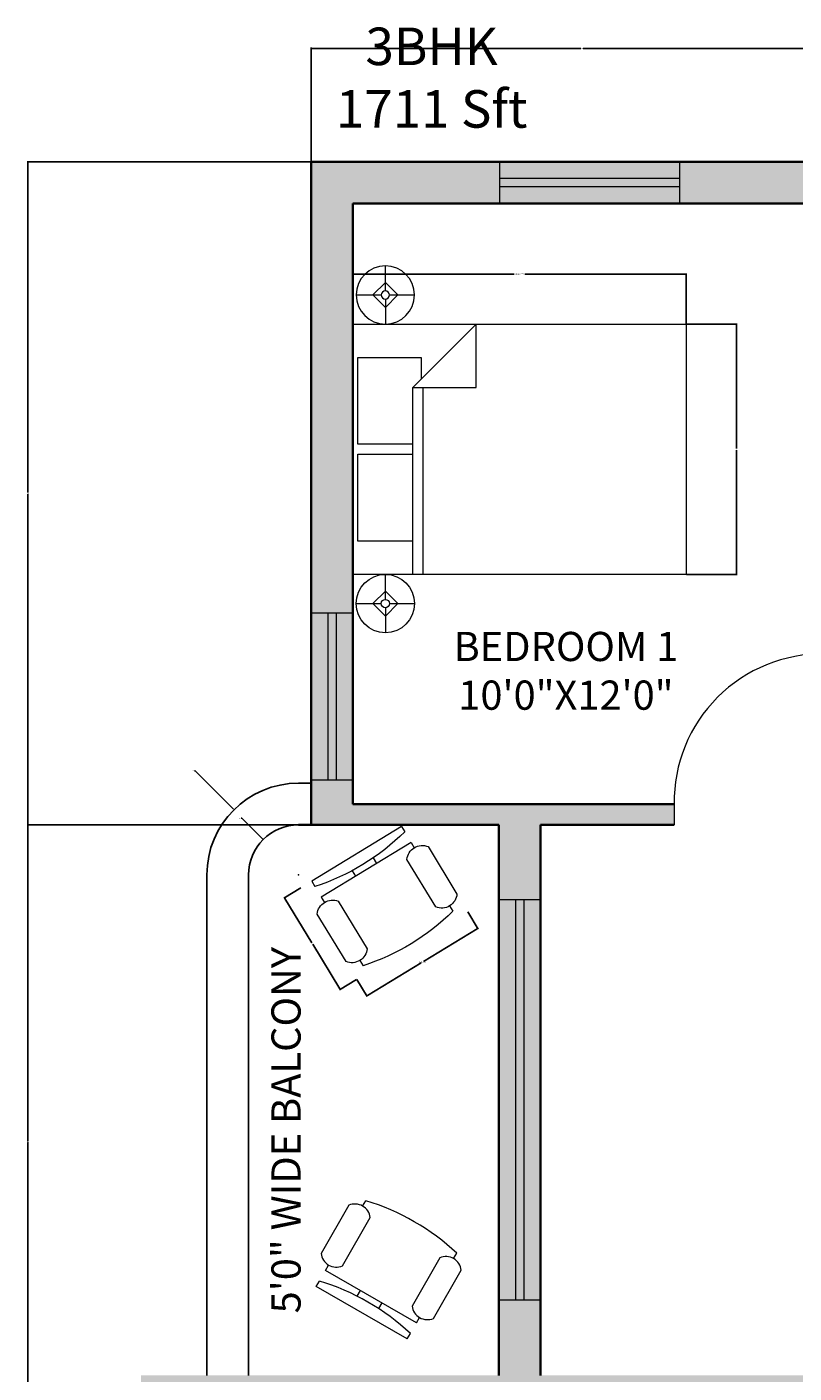
# Model space of a CAD drawing. Units: inches. Extents: x -382 to 250, y 518 to 1732.
# Tile 6 of 8: x -270 to -86, y 1373 to 1695. Entities that reach past the tile are written whole.
import ezdxf

# ---------------------------------------------------------------- set-up
doc = ezdxf.new("R2010")
doc.units = ezdxf.units.IN
doc.header["$MEASUREMENT"] = 0
for name, color, linetype, lineweight in [('A-ANNO-DIMS', 2, 'Continuous', 18), ('A-ANNO-TEXT', 7, 'Continuous', 25), ('A-AREA-IDEN', 7, 'Continuous', 18), ('A-DOOR', 3, 'Continuous', 18), ('A-FLOR-EDGE', 7, 'Continuous', 25), ('A-FURN', 8, 'Continuous', 18), ('A-GLAZ', 4, 'Continuous', 18), ('A-WALL', 7, 'Continuous', 35)]:
    doc.layers.add(name, color=color, linetype=linetype, lineweight=lineweight)
doc.layers.add('A-GLAZ-PATT', color=143, linetype='Continuous', lineweight=13, true_color=0x7aafdf)
doc.layers.add('A-WALL-PATT', color=251, linetype='Continuous', lineweight=13, true_color=0x636466)
doc.styles.get("Standard").update_dxf_attribs({"font": 'arial.ttf'})
doc.dimstyles.get("Standard").update_dxf_attribs({"dimtxt": 0.18, "dimasz": 0.18, "dimexe": 0.18, "dimexo": 0.0625, "dimgap": 0.09, "dimtad": 0, "dimtih": 1, "dimtoh": 1, "dimdec": 4, "dimzin": 0, "dimdsep": 46, "dimtxsty": 'Standard', "dimcen": 0.09, "dimadec": 0, "dimazin": 0, "dimtfac": 1, "dimtdec": 4, "dimtofl": 0, "dimtmove": 0, "dimatfit": 3, "dimfxl": 1, "dimtolj": 1, "dimtzin": 0, "dimarcsym": 0})

# ---------------------------------------------------------------- blocks, each defined once
blk = doc.blocks.new('Bed - Queen')
for p, q in [((0, -80.00003), (0, 0)), ((0, 0), (59.99999, 0)), ((59.99999, 0), (59.99999, -80.00003)), ((7.99999, -1.2), (28.79998, -1.2)), ((7.99999, -14.4), (7.99999, -1.2)), ((28.79998, -1.2), (28.79998, -14.4)), ((31.19999, -1.2), (51.99999, -1.2)), ((31.19999, -14.4), (31.19999, -1.2)), ((51.99999, -1.2), (51.99999, -16.4)), ((0, -14.4), (44.8, -14.4)), ((59.99999, -29.6), (44.8, -14.4)), ((44.8, -14.4), (44.8, -29.6)), ((44.8, -16.8), (0, -16.8)), ((51.99999, -16.4), (46.79936, -16.4)), ((44.8, -29.6), (59.99999, -29.6)), ((59.99999, -80.00003), (0, -80.00003))]:
    blk.add_line(p, q)
blk = doc.blocks.new('Lamp - Table')
for p, q in [((0, 7), (0, 1)), ((-1, 0), (-7, 0)), ((0, 3), (-3, 0)), ((-3, 0), (0, -3)), ((3, 0), (0, 3)), ((0, -3), (3, 0)), ((1, 0), (7, 0)), ((0, -1), (0, -7))]:
    blk.add_line(p, q)
for radius in [7, 1]:
    blk.add_circle((0, 0), radius)
blk = doc.blocks.new('Chair - Desk')
for p, q in [((-8.5, 0), (-8.5, -1)), ((-8.5, 0), (8.5, 0)), ((8.5, 0), (8.5, -1)), ((-2, -3), (-2, -1.9355)), ((2, -1.9576), (2, -3)), ((-8.5, -3), (-8.5, -4)), ((-8.5, -3), (8.5, -3)), ((8.5, -3), (8.5, -4)), ((-10.5, -5), (-10.5, -14)), ((-6.5, -14), (-6.5, -5)), ((6.5, -5), (6.5, -14)), ((10.5, -14), (10.5, -5)), ((-8.5, -15), (-8.5, -16)), ((8.5, -15), (8.5, -16))]:
    blk.add_line(p, q)
for centre, radius, start, end in [((0, 34.625), 36.625, 256.5803, 283.4197), ((-8.5, -6.5), 2.5, 36.8699, 143.1301), ((8.5, -6.5), 2.5, 36.8699, 143.1301), ((-8.5, -12.5), 2.5, 216.8699, 323.1301), ((8.5, -12.5), 2.5, 216.8699, 323.1301), ((0, 19.625), 36.625, 256.5803, 283.4197)]:
    blk.add_arc(centre, radius, start, end)
blk = doc.blocks.new('WIN-43_2IN')
for p, q in [((0, 10), (0, 0)), ((43.2, 10), (43.2, 0)), ((0, 6), (43.2, 6)), ((0, 4), (43.2, 4))]:
    blk.add_line(p, q)
blk = doc.blocks.new('WIN-40IN')
for p, q in [((10, 40), (0, 40)), ((4, 40), (4, 0)), ((6, 40), (6, 0)), ((10, 0), (0, 0))]:
    blk.add_line(p, q)
blk = doc.blocks.new('DOOR-SWING-36IN')
for p, q in [((-1, 0), (-1, 36)), ((0, 0), (0, 36))]:
    blk.add_line(p, q)
blk.add_arc((-0.5, 0.5), 35.5, 89.1931, 180.8069)
blk = doc.blocks.new('GLAZ-BALCONY-96IN')
for p, q in [((0, 10), (0, 0)), ((96, 10), (96, 0)), ((0, 6), (96, 6)), ((0, 4), (96, 4))]:
    blk.add_line(p, q)
blk = doc.blocks.new('*D28')
at = {"layer": 'A-ANNO-DIMS', "color": 0, "lineweight": -2, "transparency": 16777216}
for p, q in [((-192.22, 1624.2), (-192.22, 1636.31)), ((-192.04, 1636.13), (-153.52, 1636.13)), ((-112.39, 1636.13), (-150.91, 1636.13)), ((-112.21, 1624.2), (-112.21, 1636.31))]:
    blk.add_line(p, q, dxfattribs=at)
at = {"layer": 'A-ANNO-DIMS', "color": 0, "transparency": 16777216}
for points in [[(-192.04, 1636.16), (-192.04, 1636.1), (-192.22, 1636.13)], [(-112.39, 1636.16), (-112.39, 1636.1), (-112.21, 1636.13)]]:
    blk.add_solid(points, dxfattribs=at)
at = {"layer": 'Defpoints', "color": 0, "transparency": 16777216}
for p in [(-192.22, 1636.13), (-192.22, 1624.13), (-112.21, 1624.13)]:
    blk.add_point(p, dxfattribs=at)
at = {"layer": 'A-ANNO-DIMS', "color": 0, "transparency": 16777216, "insert": (-152.22, 1636.13), "char_height": 0.18, "attachment_point": 5}
blk.add_mtext('\\A1;QUEEN BED 80 TYP.', dxfattribs=at)
blk = doc.blocks.new('*D29')
at = {"layer": 'A-ANNO-DIMS', "color": 0, "lineweight": -2, "transparency": 16777216}
for p, q in [((-112.15, 1624.13), (-100.03, 1624.13)), ((-100.21, 1623.95), (-100.21, 1594.32)), ((-100.21, 1564.31), (-100.21, 1593.95)), ((-112.15, 1564.13), (-100.03, 1564.13))]:
    blk.add_line(p, q, dxfattribs=at)
at = {"layer": 'A-ANNO-DIMS', "color": 0, "transparency": 16777216}
for points in [[(-100.24, 1623.95), (-100.18, 1623.95), (-100.21, 1624.13)], [(-100.24, 1564.31), (-100.18, 1564.31), (-100.21, 1564.13)]]:
    blk.add_solid(points, dxfattribs=at)
at = {"layer": 'Defpoints', "color": 0, "transparency": 16777216}
for p in [(-112.21, 1624.13), (-100.21, 1624.13), (-112.21, 1564.13)]:
    blk.add_point(p, dxfattribs=at)
at = {"layer": 'A-ANNO-DIMS', "color": 0, "transparency": 16777216, "insert": (-100.21, 1594.13), "char_height": 0.18, "attachment_point": 5}
blk.add_mtext('\\A1;60 TYP.', dxfattribs=at)
blk = doc.blocks.new('*D38')
at = {"layer": 'A-ANNO-DIMS', "color": 0, "lineweight": -2, "transparency": 16777216}
for p, q in [((-164.62, 1483.19), (-162.13, 1479.09)), ((-162.38, 1479.15), (-175.23, 1471.34)), ((-188.68, 1463.16), (-175.83, 1470.98)), ((-191.22, 1467.01), (-188.74, 1462.92))]:
    blk.add_line(p, q, dxfattribs=at)
at = {"layer": 'A-ANNO-DIMS', "color": 0, "transparency": 16777216}
for points in [[(-162.4, 1479.18), (-162.36, 1479.13), (-162.23, 1479.25)], [(-188.69, 1463.19), (-188.66, 1463.14), (-188.83, 1463.07)]]:
    blk.add_solid(points, dxfattribs=at)
at = {"layer": 'Defpoints', "color": 0, "transparency": 16777216}
for p in [(-164.65, 1483.24), (-191.26, 1467.06), (-188.83, 1463.07)]:
    blk.add_point(p, dxfattribs=at)
at = {"layer": 'A-ANNO-DIMS', "color": 0, "transparency": 16777216, "insert": (-175.53, 1471.16), "char_height": 0.18, "attachment_point": 5}
blk.add_mtext('\\A1;CHAIR 31 TYP.', dxfattribs=at)
blk = doc.blocks.new('*D39')
at = {"layer": 'A-ANNO-DIMS', "color": 0, "lineweight": -2, "transparency": 16777216}
for p, q in [((-204.66, 1488.99), (-208.75, 1486.5)), ((-208.51, 1486.44), (-202.03, 1475.8)), ((-195.34, 1464.79), (-201.81, 1475.43)), ((-191.31, 1467.03), (-195.4, 1464.54))]:
    blk.add_line(p, q, dxfattribs=at)
at = {"layer": 'A-ANNO-DIMS', "color": 0, "transparency": 16777216}
for points in [[(-208.48, 1486.46), (-208.53, 1486.42), (-208.6, 1486.59)], [(-195.32, 1464.8), (-195.37, 1464.77), (-195.25, 1464.63)]]:
    blk.add_solid(points, dxfattribs=at)
at = {"layer": 'Defpoints', "color": 0, "transparency": 16777216}
for p in [(-204.61, 1489.02), (-208.6, 1486.59), (-191.26, 1467.06)]:
    blk.add_point(p, dxfattribs=at)
at = {"layer": 'A-ANNO-DIMS', "color": 0, "transparency": 16777216, "insert": (-201.92, 1475.61), "char_height": 0.18, "attachment_point": 5}
blk.add_mtext('\\A1;26 TYP.', dxfattribs=at)
blk = doc.blocks.new('*D88')
at = {"layer": 'A-ANNO-DIMS', "color": 0, "lineweight": -2, "transparency": 16777216}
for p, q in [((-202.22, 1663.13), (-202.22, 1690.45)), ((-202.04, 1690.27), (-137.5, 1690.27)), ((-72.4, 1690.27), (-136.93, 1690.27)), ((-72.22, 1663.13), (-72.22, 1690.45))]:
    blk.add_line(p, q, dxfattribs=at)
at = {"layer": 'A-ANNO-DIMS', "color": 0, "transparency": 16777216}
for points in [[(-202.04, 1690.3), (-202.04, 1690.24), (-202.22, 1690.27)], [(-72.4, 1690.3), (-72.4, 1690.24), (-72.22, 1690.27)]]:
    blk.add_solid(points, dxfattribs=at)
at = {"layer": 'Defpoints', "color": 0, "transparency": 16777216}
for p in [(-72.22, 1690.27), (-202.22, 1663.07), (-72.22, 1663.07)]:
    blk.add_point(p, dxfattribs=at)
at = {"layer": 'A-ANNO-DIMS', "color": 0, "transparency": 16777216, "insert": (-137.22, 1690.27), "char_height": 0.18, "attachment_point": 5}
blk.add_mtext('\\A1;130', dxfattribs=at)
blk = doc.blocks.new('*D92')
at = {"layer": 'A-ANNO-DIMS', "color": 0, "lineweight": -2, "transparency": 16777216}
for p, q in [((-202.28, 1504.07), (-270.36, 1504.07)), ((-270.18, 1503.89), (-270.18, 1428.25)), ((-270.18, 1352.25), (-270.18, 1427.89)), ((-243.04, 1352.07), (-270.36, 1352.07))]:
    blk.add_line(p, q, dxfattribs=at)
at = {"layer": 'A-ANNO-DIMS', "color": 0, "transparency": 16777216}
for points in [[(-270.21, 1503.89), (-270.15, 1503.89), (-270.18, 1504.07)], [(-270.21, 1352.25), (-270.15, 1352.25), (-270.18, 1352.07)]]:
    blk.add_solid(points, dxfattribs=at)
at = {"layer": 'Defpoints', "color": 0, "transparency": 16777216}
for p in [(-270.18, 1504.07), (-202.22, 1504.07), (-242.98, 1352.07)]:
    blk.add_point(p, dxfattribs=at)
at = {"layer": 'A-ANNO-DIMS', "color": 0, "transparency": 16777216, "insert": (-270.18, 1428.07), "char_height": 0.18, "attachment_point": 5}
blk.add_mtext('\\A1;152', dxfattribs=at)
blk = doc.blocks.new('*D93')
at = {"layer": 'A-ANNO-DIMS', "color": 0, "lineweight": -2, "transparency": 16777216}
for p, q in [((-202.28, 1663.07), (-270.36, 1663.07)), ((-270.18, 1662.89), (-270.18, 1583.75)), ((-270.18, 1504.25), (-270.18, 1583.39)), ((-202.28, 1504.07), (-270.36, 1504.07))]:
    blk.add_line(p, q, dxfattribs=at)
at = {"layer": 'A-ANNO-DIMS', "color": 0, "transparency": 16777216}
for points in [[(-270.21, 1662.89), (-270.15, 1662.89), (-270.18, 1663.07)], [(-270.21, 1504.25), (-270.15, 1504.25), (-270.18, 1504.07)]]:
    blk.add_solid(points, dxfattribs=at)
at = {"layer": 'Defpoints', "color": 0, "transparency": 16777216}
for p in [(-270.18, 1663.07), (-202.22, 1663.07), (-202.22, 1504.07)]:
    blk.add_point(p, dxfattribs=at)
at = {"layer": 'A-ANNO-DIMS', "color": 0, "transparency": 16777216, "insert": (-270.18, 1583.57), "char_height": 0.18, "attachment_point": 5}
blk.add_mtext('\\A1;159', dxfattribs=at)
blk = doc.blocks.new('*D98')
at = {"layer": 'A-ANNO-DIMS', "color": 0, "lineweight": -2, "transparency": 16777216}
for p, q in [((-230.17, 1517.07), (-229.99, 1517.07)), ((-229.99, 1517.07), (-220.83, 1507.82)), ((-205.31, 1492.07), (-205.13, 1492.07)), ((-205.22, 1491.98), (-205.22, 1492.16))]:
    blk.add_line(p, q, dxfattribs=at)
at = {"layer": 'A-ANNO-DIMS', "color": 0, "transparency": 16777216}
blk.add_solid([(-220.8, 1507.85), (-220.85, 1507.8), (-220.7, 1507.7)], dxfattribs=at)
at = {"layer": 'Defpoints', "color": 0, "transparency": 16777216}
for p in [(-220.7, 1507.7), (-205.22, 1492.07)]:
    blk.add_point(p, dxfattribs=at)
at = {"layer": 'A-ANNO-DIMS', "color": 0, "transparency": 16777216, "insert": (-230.47, 1517.07), "char_height": 0.18, "attachment_point": 5}
blk.add_mtext('\\A1;R22', dxfattribs=at)
blk = doc.blocks.new('*D99')
at = {"layer": 'A-ANNO-DIMS', "color": 0, "lineweight": -2, "transparency": 16777216}
for p, q in [((-218.97, 1505.65), (-218.79, 1505.65)), ((-218.79, 1505.65), (-213.83, 1500.68)), ((-205.31, 1492.07), (-205.13, 1492.07)), ((-205.22, 1491.98), (-205.22, 1492.16))]:
    blk.add_line(p, q, dxfattribs=at)
at = {"layer": 'A-ANNO-DIMS', "color": 0, "transparency": 16777216}
blk.add_solid([(-213.81, 1500.7), (-213.85, 1500.66), (-213.7, 1500.55)], dxfattribs=at)
at = {"layer": 'Defpoints', "color": 0, "transparency": 16777216}
for p in [(-213.7, 1500.55), (-205.22, 1492.07)]:
    blk.add_point(p, dxfattribs=at)
at = {"layer": 'A-ANNO-DIMS', "color": 0, "transparency": 16777216, "insert": (-219.28, 1505.65), "char_height": 0.18, "attachment_point": 5}
blk.add_mtext('\\A1;R12', dxfattribs=at)

msp = doc.modelspace()

# ---------------------------------------------------------------- hatches: boundary and pattern name
at = {"layer": 'A-GLAZ-PATT'}
h = msp.add_hatch(color=256, dxfattribs=at)
h.dxf.hatch_style = 1
h.paths.add_polyline_path([(-113.7732, 1663.0687), (-156.9732, 1663.0687), (-156.9732, 1659.0687), (-113.7732, 1659.0687)])
h = msp.add_hatch(color=256, dxfattribs=at)
h.dxf.hatch_style = 1
h.paths.add_polyline_path([(-113.7732, 1659.0687), (-156.9732, 1659.0687), (-156.9732, 1657.0687), (-113.7732, 1657.0687)])
h = msp.add_hatch(color=256, dxfattribs=at)
h.dxf.hatch_style = 1
h.paths.add_polyline_path([(-113.7732, 1657.0687), (-156.9732, 1657.0687), (-156.9732, 1653.0687), (-113.7732, 1653.0687)])
h = msp.add_hatch(color=256, dxfattribs=at)
h.dxf.hatch_style = 1
h.paths.add_polyline_path([(-198.215, 1554.8323), (-202.215, 1554.8323), (-202.215, 1514.8323), (-198.215, 1514.8323)])
h = msp.add_hatch(color=256, dxfattribs=at)
h.dxf.hatch_style = 1
h.paths.add_polyline_path([(-196.215, 1554.8323), (-198.215, 1554.8323), (-198.215, 1514.8323), (-196.215, 1514.8323)])
h = msp.add_hatch(color=256, dxfattribs=at)
h.dxf.hatch_style = 1
h.paths.add_polyline_path([(-192.215, 1554.8323), (-196.215, 1554.8323), (-196.215, 1514.8323), (-192.215, 1514.8323)])
h = msp.add_hatch(color=256, dxfattribs=at)
h.dxf.hatch_style = 1
h.paths.add_polyline_path([(-153.215, 1486.0687), (-157.215, 1486.0687), (-157.215, 1390.0687), (-153.215, 1390.0687)])
h = msp.add_hatch(color=256, dxfattribs=at)
h.dxf.hatch_style = 1
h.paths.add_polyline_path([(-151.215, 1486.0687), (-153.215, 1486.0687), (-153.215, 1390.0687), (-151.215, 1390.0687)])
h = msp.add_hatch(color=256, dxfattribs=at)
h.dxf.hatch_style = 1
h.paths.add_polyline_path([(-147.215, 1486.0687), (-151.215, 1486.0687), (-151.215, 1390.0687), (-147.215, 1390.0687)])
at = {"layer": 'A-WALL-PATT'}
h = msp.add_hatch(color=256, dxfattribs=at)
h.dxf.hatch_style = 1
h.paths.add_polyline_path([(-62.215, 1653.0687), (-59.1064, 1653.0687), (-59.1064, 1663.0687), (-65.0078, 1663.0687), (-65.0078, 1680.4388), (-72.215, 1680.4388), (-72.215, 1663.0687), (-113.7732, 1663.0687), (-113.7732, 1653.0687), (-72.215, 1653.0687), (-72.215, 1582.6793), (-62.215, 1582.6793)])
h = msp.add_hatch(color=256, dxfattribs=at)
h.dxf.hatch_style = 1
h.paths.add_polyline_path([(-192.215, 1653.0687), (-156.9732, 1653.0687), (-156.9732, 1663.0687), (-202.215, 1663.0687), (-202.215, 1554.8323), (-192.215, 1554.8323)])
h = msp.add_hatch(color=256, dxfattribs=at)
h.dxf.hatch_style = 1
h.paths.add_polyline_path([(-115.1204, 1509.0687), (-192.215, 1509.0687), (-192.215, 1514.8323), (-202.215, 1514.8323), (-202.215, 1504.0687), (-157.215, 1504.0687), (-157.215, 1486.0687), (-147.215, 1486.0687), (-147.215, 1504.0687), (-115.1204, 1504.0687)])
h = msp.add_hatch(color=256, dxfattribs=at)
h.dxf.hatch_style = 1
h.paths.add_polyline_path([(-147.215, 1390.0687), (-157.215, 1390.0687), (-157.215, 1372.0687), (-217.215, 1372.0687), (-242.9787, 1372.0687), (-242.9787, 1352.0687), (-202.215, 1352.0687), (-202.215, 1341.5341), (-192.215, 1341.5341), (-192.215, 1367.0687), (-67.1575, 1367.0687), (-67.1575, 1372.0687), (-147.215, 1372.0687)])

# ---------------------------------------------------------------- linework, layer by layer
at = {"layer": 'A-DOOR'}
msp.add_line((-115.1204, 1509.0687), (-115.1204, 1504.0687), dxfattribs=at)
at = {"layer": 'A-FLOR-EDGE'}
for p, q in [((-205.215, 1514.0687), (-202.215, 1514.0687)), ((-227.215, 1492.0687), (-227.215, 1372.0687)), ((-217.215, 1492.0687), (-217.215, 1372.0687))]:
    msp.add_line(p, q, dxfattribs=at)
for radius in [22, 12]:
    msp.add_arc((-205.215, 1492.0687), radius, 90, 180, dxfattribs=at)
at = {"layer": 'A-WALL'}
for p, q in [((-72.215, 1663.0687), (-202.215, 1663.0687)), ((-202.215, 1663.0687), (-202.215, 1504.0687)), ((-192.215, 1653.0687), (-192.215, 1509.0687)), ((-72.215, 1653.0687), (-192.215, 1653.0687)), ((-192.215, 1509.0687), (-115.1204, 1509.0687)), ((-205.215, 1504.0687), (-157.215, 1504.0687)), ((-157.215, 1504.0687), (-157.215, 1372.0687)), ((-147.215, 1504.0687), (-147.215, 1372.0687)), ((-147.215, 1504.0687), (-115.1204, 1504.0687))]:
    msp.add_line(p, q, dxfattribs=at)

# ---------------------------------------------------------------- block references
at = {"layer": 'A-DOOR'}
msp.add_blockref('DOOR-SWING-36IN', (-79.1204, 1509.0687), dxfattribs=at)
at = {"layer": 'A-FURN', "xscale": -1, "rotation": 90}
msp.add_blockref('Lamp - Table', (-184.4036, 1631.1344), dxfattribs=at)
at = {"layer": 'A-FURN', "rotation": 90}
for name, p in [('Bed - Queen', (-192.215, 1564.1344)), ('Lamp - Table', (-184.4036, 1557.1344))]:
    msp.add_blockref(name, p, dxfattribs=at)
at = {"layer": 'A-FURN', "yscale": 1.482721811849832, "zscale": 1.482721811849832}
for p, xscale, rotation in [((-191.3076, 1497.1094), -1.482721811849832, 31.30212076045902), ((-190.0574, 1387.0941), 1.482721811849832, 149.9999999999999)]:
    msp.add_blockref('Chair - Desk', p, dxfattribs=dict(at, xscale=xscale, rotation=rotation))
at = {"layer": 'A-GLAZ'}
for name, p, rotation in [('WIN-43_2IN', (-113.7732, 1663.0684), 180), ('GLAZ-BALCONY-96IN', (-157.2147, 1486.0687), 270.0000000000002)]:
    msp.add_blockref(name, p, dxfattribs=dict(at, rotation=rotation))
msp.add_blockref('WIN-40IN', (-202.215, 1514.8319), dxfattribs=at)

# ---------------------------------------------------------------- texts
at = {"layer": 'A-ANNO-TEXT', "insert": (-236.8768, 1695.2539), "char_height": 9, "attachment_point": 1}
msp.add_mtext_dynamic_manual_height_columns('\\pxqc;3BHK\\P1711 Sft', width=127.14497, gutter_width=1, heights=[0], dxfattribs=at)
at = {"layer": 'A-AREA-IDEN', "insert": (-180.9133, 1550.3516), "char_height": 7, "attachment_point": 1}
msp.add_mtext_dynamic_manual_height_columns('\\pxqc;BEDROOM 1\\P10\'0"X12\'0"', width=79.656175, gutter_width=1, heights=[0], dxfattribs=at)
at = {"layer": 'A-AREA-IDEN', "insert": (-223.3991, 1379.8709), "char_height": 7, "attachment_point": 1, "rotation": 90}
msp.add_mtext_dynamic_manual_height_columns('\\pxqc;\\P5\'0" WIDE BALCONY', width=101.975496, gutter_width=1, heights=[0], dxfattribs=at)

# ---------------------------------------------------------------- dimensions: what is measured, and where the dimension line sits
at = {"layer": 'A-ANNO-DIMS'}
dim = msp.add_linear_dim(base=(-72.215, 1690.2687), p1=(-202.215, 1663.0687), p2=(-72.215, 1663.0687), dimstyle='Standard', override={"dimdec": 0, "dimlfac": 1, "dimrnd": 0, "dimzin": 0, "dimdsep": 46, "dimlunit": 2}, dxfattribs=at)
dim.commit()
dim.dimension.update_dxf_attribs({"geometry": '*D88', "text_midpoint": (-137.215, 1690.2687)})
for base, p1, p2, picture, middle in [((-270.1787, 1663.0687), (-202.215, 1504.0687), (-202.215, 1663.0687), '*D93', (-270.1787, 1583.5687)), ((-270.1787, 1504.0687), (-242.9787, 1352.0687), (-202.215, 1504.0687), '*D92', (-270.1787, 1428.0687))]:
    dim = msp.add_linear_dim(base=base, p1=p1, p2=p2, angle=90, dimstyle='Standard', override={"dimdec": 0, "dimlfac": 1, "dimrnd": 0, "dimzin": 0, "dimdsep": 46, "dimlunit": 2}, dxfattribs=at)
    dim.commit()
    dim.dimension.update_dxf_attribs({"geometry": picture, "text_midpoint": middle})
for base, p1, p2, angle, text, picture, middle in [((-192.215, 1636.1344), (-112.215, 1624.1344), (-192.215, 1624.1344), 180, 'QUEEN BED <> TYP.', '*D28', (-152.215, 1636.1344)), ((-100.215, 1624.1344), (-112.215, 1564.1344), (-112.215, 1624.1344), 90, '<> TYP.', '*D29', (-100.215, 1594.1344)), ((-208.6007, 1486.5941), (-191.2573, 1467.0612), (-204.61, 1489.0207), 121.302121, '<> TYP.', '*D39', (-201.9243, 1475.6143)), ((-188.8307, 1463.0704), (-164.6524, 1483.2385), (-191.2573, 1467.0612), 211.302121, 'CHAIR <> TYP.', '*D38', (-175.5282, 1471.1591))]:
    dim = msp.add_linear_dim(base=base, p1=p1, p2=p2, angle=angle, text=text, dimstyle='Standard', override={"dimdec": 0, "dimlfac": 1, "dimrnd": 0, "dimzin": 0, "dimdsep": 46, "dimlunit": 2}, dxfattribs=at)
    dim.commit()
    dim.dimension.update_dxf_attribs({"geometry": picture, "text_midpoint": middle})
for mpoint, picture, middle in [((-220.6994, 1507.6967), '*D98', (-230.4742, 1517.0734)), ((-213.7001, 1500.5541), '*D99', (-219.2753, 1505.6454))]:
    dim = msp.add_radius_dim(center=(-205.215, 1492.0687), mpoint=mpoint, dimstyle='Standard', override={"dimdec": 0, "dimlfac": 1, "dimrnd": 0, "dimzin": 0, "dimdsep": 46, "dimlunit": 2}, dxfattribs=at)
    dim.commit()
    dim.dimension.update_dxf_attribs({"geometry": picture, "text_midpoint": middle, "dimtype": 164})

doc.saveas('drawing.dxf')
